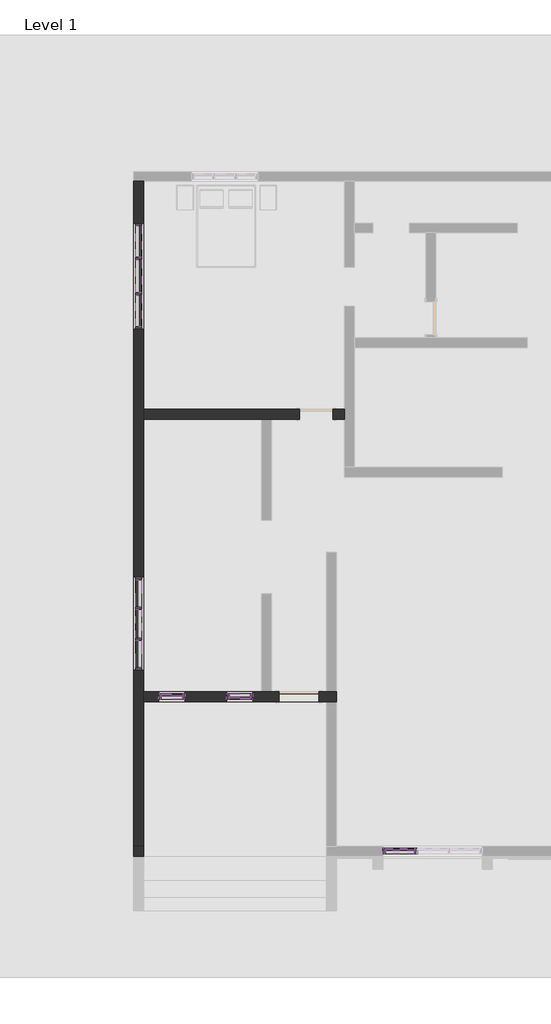
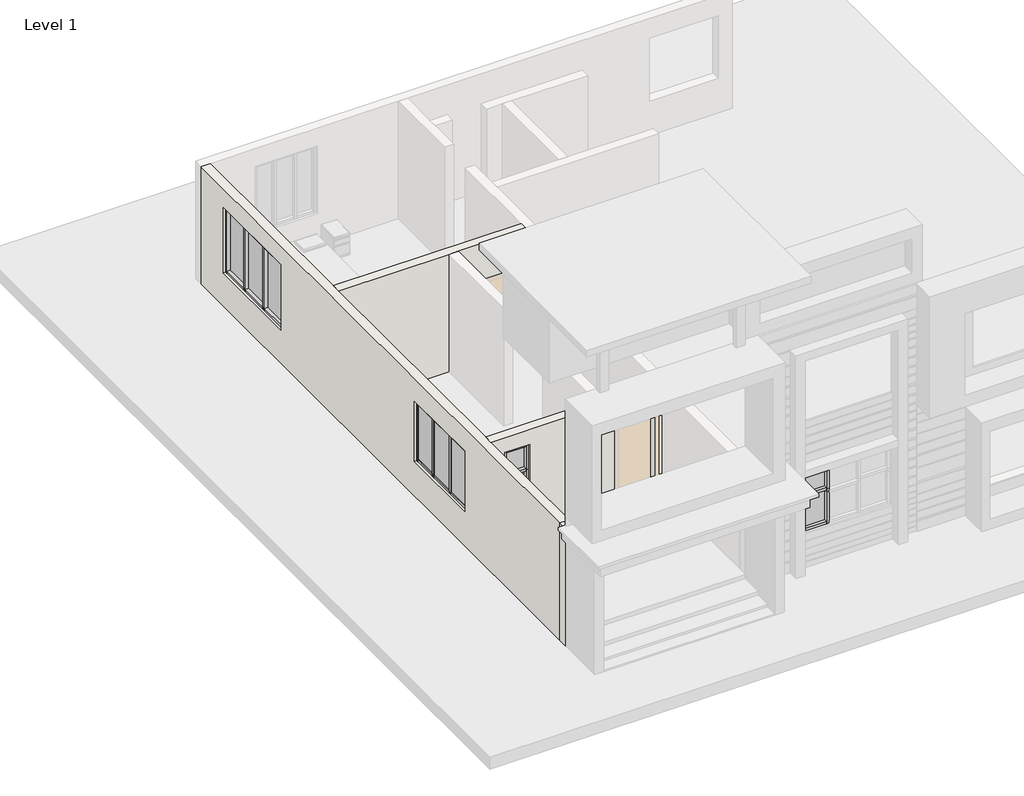
# One storey, part 1 of 3: 49 members, 14 plates, 4 walls.
"""IFC4 building model written with IfcOpenShell, lengths in millimetres."""

from ifc_helpers import new_model, si_unit, origin, origin_with_axes, place, context, project, spatial, polyline, outline, extrude, faceted_brep, transform, mapped, element, save
from components import member_9d02be77, member_7007ad49, member_4a676c08, member_d25e63f8, member_22561c7a, member_3f0e0172, member_607f7529, member_5215b92c, member_00d00b53, member_eb7364f1, member_5ab2641c, member_2ee2964b, member_c33c434a, member_3d7cb871, member_24f36acb, member_a6ee1c2c, member_c4c38143, member_86d06fe4, member_323df77c, member_e6bcc2de, system_panel_glazed_30ed1ba4, system_panel_glazed_23add07f, system_panel_glazed_742ba722, system_panel_glazed_f4631ac9, system_panel_glazed_21711ca4, system_panel_glazed_687c427d, system_panel_glazed_19f1df67, system_panel_glazed_625789f6, system_panel_glazed_f3433a31, system_panel_glazed_9cf13bc3

model = new_model("IFC4")

# Units and contexts
model_context = context("Model", 3, world=origin())
ifc_project = project(units=[si_unit("LENGTHUNIT", "METRE", prefix="MILLI")], contexts=[model_context])

# Site, building, storey
site = spatial("IfcSite", under=ifc_project)
building = spatial("IfcBuilding", under=site)
storey = spatial("IfcBuildingStorey", under=building, Name="Level 1", Elevation=0.0)

# Members
placement = place(None, origin())
member_shape = member_9d02be77(model_context)
element("IfcMember", 1, ObjectType="Rectangular Mullion : 2.5\" x 5\" rectangular", at=placement, inside=storey, context=model_context, shape_type="MappedRepresentation", body=[
    mapped(member_shape, transform((-18686.1761094, -1937.896149, 2567.6785541), x_axis=(0.0, 0.0, 1.0), y_axis=(-1.0, 0.0, 0.0), z_axis=(0.0, -1.0, 0.0))),
])
member_2_shape = member_7007ad49(model_context)
element("IfcMember", 2, ObjectType="Rectangular Mullion : 2.5\" x 5\" rectangular", at=placement, inside=storey, context=model_context, shape_type="MappedRepresentation", body=[
    mapped(member_2_shape, transform((-18686.1761094, -1125.096149, 2567.6785541), x_axis=(0.0, 0.0, 1.0), y_axis=(-1.0, 0.0, 0.0), z_axis=(0.0, -1.0, 0.0))),
])
element("IfcMember", 3, ObjectType="Rectangular Mullion : 2.5\" x 5\" rectangular", at=placement, inside=storey, context=model_context, shape_type="MappedRepresentation", body=[
    mapped(member_2_shape, transform((-18686.1761094, -2718.946149, 2567.6785541), x_axis=(0.0, 0.0, 1.0), y_axis=(-1.0, 0.0, 0.0), z_axis=(0.0, -1.0, 0.0))),
])
member_3_shape = member_4a676c08(model_context)
element("IfcMember", 4, ObjectType="Rectangular Mullion : 2.5\" x 5\" rectangular", at=placement, inside=storey, context=model_context, shape_type="MappedRepresentation", body=[
    mapped(member_3_shape, transform((-18686.1761094, -1969.646149, 870.2260305), x_axis=(0.0, -1.0, 0.0), y_axis=(-1.0, 0.0, 0.0), z_axis=(0.0, 0.0, -1.0))),
])
element("IfcMember", 5, ObjectType="Rectangular Mullion : 2.5\" x 5\" rectangular", at=placement, inside=storey, context=model_context, shape_type="MappedRepresentation", body=[
    mapped(member_3_shape, transform((-18686.1761094, -1156.846149, 870.2260305), x_axis=(0.0, -1.0, 0.0), y_axis=(-1.0, 0.0, 0.0), z_axis=(0.0, 0.0, -1.0))),
])
element("IfcMember", 6, ObjectType="Rectangular Mullion : 2.5\" x 5\" rectangular", at=placement, inside=storey, context=model_context, shape_type="MappedRepresentation", body=[
    mapped(member_2_shape, transform((-18686.1761094, -2001.396149, 870.2260305), x_axis=(0.0, 0.0, -1.0), y_axis=(-1.0, 0.0, 0.0), z_axis=(0.0, 1.0, 0.0))),
])
element("IfcMember", 7, ObjectType="Rectangular Mullion : 2.5\" x 5\" rectangular", at=placement, inside=storey, context=model_context, shape_type="MappedRepresentation", body=[
    mapped(member_2_shape, transform((-18686.1761094, -407.546149, 870.2260305), x_axis=(0.0, 0.0, -1.0), y_axis=(-1.0, 0.0, 0.0), z_axis=(0.0, 1.0, 0.0))),
])
element("IfcMember", 8, ObjectType="Rectangular Mullion : 2.5\" x 5\" rectangular", at=placement, inside=storey, context=model_context, shape_type="MappedRepresentation", body=[
    mapped(member_shape, transform((-18686.1761094, -1188.596149, 870.2260305), x_axis=(0.0, 0.0, -1.0), y_axis=(-1.0, 0.0, 0.0), z_axis=(0.0, 1.0, 0.0))),
])
member_4_shape = member_d25e63f8(model_context)
element("IfcMember", 9, ObjectType="Rectangular Mullion : 2.5\" x 5\" rectangular", at=placement, inside=storey, context=model_context, shape_type="MappedRepresentation", body=[
    mapped(member_4_shape, transform((-18686.1761094, -2782.446149, 870.2260305), x_axis=(0.0, -1.0, 0.0), y_axis=(-1.0, 0.0, 0.0), z_axis=(0.0, 0.0, -1.0))),
])
element("IfcMember", 10, ObjectType="Rectangular Mullion : 2.5\" x 5\" rectangular", at=placement, inside=storey, context=model_context, shape_type="MappedRepresentation", body=[
    mapped(member_4_shape, transform((-18686.1761094, -344.046149, 2567.6785541), x_axis=(0.0, 1.0, 0.0), y_axis=(-1.0, 0.0, 0.0), z_axis=(0.0, 0.0, 1.0))),
])
member_5_shape = member_22561c7a(model_context)
element("IfcMember", 11, ObjectType="Rectangular Mullion : 2.5\" x 5\" rectangular", at=placement, inside=storey, context=model_context, shape_type="MappedRepresentation", body=[
    mapped(member_5_shape, transform((-18686.1761094, -10592.946149, 2458.72085), x_axis=(0.0, -1.0, 0.0), y_axis=(1.0, 0.0, 0.0), z_axis=(0.0, 0.0, 1.0))),
])
member_6_shape = member_3f0e0172(model_context)
element("IfcMember", 12, ObjectType="Rectangular Mullion : 2.5\" x 5\" rectangular", at=placement, inside=storey, context=model_context, shape_type="MappedRepresentation", body=[
    mapped(member_6_shape, transform((-18686.1761094, -9913.496149, 2458.72085), x_axis=(0.0, 0.0, 1.0), y_axis=(1.0, 0.0, 0.0), z_axis=(0.0, 1.0, 0.0))),
])
element("IfcMember", 13, ObjectType="Rectangular Mullion : 2.5\" x 5\" rectangular", at=placement, inside=storey, context=model_context, shape_type="MappedRepresentation", body=[
    mapped(member_6_shape, transform((-18686.1761094, -8522.846149, 2458.72085), x_axis=(0.0, 0.0, 1.0), y_axis=(1.0, 0.0, 0.0), z_axis=(0.0, 1.0, 0.0))),
])
element("IfcMember", 14, ObjectType="Rectangular Mullion : 2.5\" x 5\" rectangular", at=placement, inside=storey, context=model_context, shape_type="MappedRepresentation", body=[
    mapped(member_6_shape, transform((-18686.1761094, -9138.796149, 901.2674751), x_axis=(0.0, 0.0, -1.0), y_axis=(1.0, 0.0, 0.0), z_axis=(0.0, -1.0, 0.0))),
])
element("IfcMember", 15, ObjectType="Rectangular Mullion : 2.5\" x 5\" rectangular", at=placement, inside=storey, context=model_context, shape_type="MappedRepresentation", body=[
    mapped(member_6_shape, transform((-18686.1761094, -10529.446149, 901.2674751), x_axis=(0.0, 0.0, -1.0), y_axis=(1.0, 0.0, 0.0), z_axis=(0.0, -1.0, 0.0))),
])
member_7_shape = member_607f7529(model_context)
element("IfcMember", 16, ObjectType="Rectangular Mullion : 2.5\" x 5\" rectangular", at=placement, inside=storey, context=model_context, shape_type="MappedRepresentation", body=[
    mapped(member_7_shape, transform((-18686.1761094, -9881.746149, 901.2674751), x_axis=(0.0, 1.0, 0.0), y_axis=(1.0, 0.0, 0.0), z_axis=(0.0, 0.0, -1.0))),
])
element("IfcMember", 17, ObjectType="Rectangular Mullion : 2.5\" x 5\" rectangular", at=placement, inside=storey, context=model_context, shape_type="MappedRepresentation", body=[
    mapped(member_7_shape, transform((-18686.1761094, -9170.546149, 901.2674751), x_axis=(0.0, 1.0, 0.0), y_axis=(1.0, 0.0, 0.0), z_axis=(0.0, 0.0, -1.0))),
])
member_8_shape = member_5215b92c(model_context)
element("IfcMember", 18, ObjectType="Rectangular Mullion : 2.5\" x 5\" rectangular", at=placement, inside=storey, context=model_context, shape_type="MappedRepresentation", body=[
    mapped(member_8_shape, transform((-18686.1761094, -9202.296149, 2458.72085), x_axis=(0.0, 0.0, 1.0), y_axis=(1.0, 0.0, 0.0), z_axis=(0.0, 1.0, 0.0))),
])
element("IfcMember", 19, ObjectType="Rectangular Mullion : 2.5\" x 5\" rectangular", at=placement, inside=storey, context=model_context, shape_type="MappedRepresentation", body=[
    mapped(member_8_shape, transform((-18686.1761094, -9849.996149, 901.2674751), x_axis=(0.0, 0.0, -1.0), y_axis=(1.0, 0.0, 0.0), z_axis=(0.0, -1.0, 0.0))),
])
element("IfcMember", 20, ObjectType="Rectangular Mullion : 2.5\" x 5\" rectangular", at=placement, inside=storey, context=model_context, shape_type="MappedRepresentation", body=[
    mapped(member_5_shape, transform((-18686.1761094, -8459.346149, 901.2674751), x_axis=(0.0, 1.0, 0.0), y_axis=(1.0, 0.0, 0.0), z_axis=(0.0, 0.0, -1.0))),
])
member_9_shape = member_00d00b53(model_context)
element("IfcMember", 21, ObjectType="Rectangular Mullion : 2.5\" x 5\" rectangular", at=placement, inside=storey, context=model_context, shape_type="MappedRepresentation", body=[
    mapped(member_9_shape, transform((-12323.9127168, -14745.846149, 1704.2081862), x_axis=(1.0, 0.0, 0.0), y_axis=(0.0, -1.0, 0.0), z_axis=(0.0, 0.0, -1.0))),
])
member_10_shape = member_eb7364f1(model_context)
element("IfcMember", 22, ObjectType="Rectangular Mullion : 2.5\" x 5\" rectangular", at=placement, inside=storey, context=model_context, shape_type="MappedRepresentation", body=[
    mapped(member_10_shape, transform((-12323.9127168, -14745.846149, 1780.4081862), x_axis=(1.0, 0.0, 0.0), y_axis=(0.0, -1.0, 0.0), z_axis=(0.0, 0.0, -1.0))),
])
member_11_shape = member_5ab2641c(model_context)
element("IfcMember", 23, ObjectType="Rectangular Mullion : 2.5\" x 5\" rectangular", at=placement, inside=storey, context=model_context, shape_type="MappedRepresentation", body=[
    mapped(member_11_shape, transform((-12323.9127168, -14745.846149, 871.6720769), x_axis=(1.0, 0.0, 0.0), y_axis=(0.0, -1.0, 0.0), z_axis=(0.0, 0.0, -1.0))),
])
member_12_shape = member_2ee2964b(model_context)
element("IfcMember", 24, ObjectType="Rectangular Mullion : 2.5\" x 5\" rectangular", at=placement, inside=storey, context=model_context, shape_type="MappedRepresentation", body=[
    mapped(member_12_shape, transform((-12355.6627168, -14745.846149, 1780.4081862), x_axis=(0.0, 0.0, 1.0), y_axis=(0.0, -1.0, 0.0), z_axis=(1.0, 0.0, 0.0))),
])
member_13_shape = member_c33c434a(model_context)
element("IfcMember", 25, ObjectType="Rectangular Mullion : 2.5\" x 5\" rectangular", at=placement, inside=storey, context=model_context, shape_type="MappedRepresentation", body=[
    mapped(member_13_shape, transform((-12355.6627168, -14745.846149, 2536.7442955), x_axis=(0.0, 0.0, 1.0), y_axis=(0.0, -1.0, 0.0), z_axis=(1.0, 0.0, 0.0))),
])
element("IfcMember", 26, ObjectType="Rectangular Mullion : 2.5\" x 5\" rectangular", at=placement, inside=storey, context=model_context, shape_type="MappedRepresentation", body=[
    mapped(member_13_shape, transform((-13022.4127168, -14745.846149, 871.6720769), x_axis=(0.0, 0.0, -1.0), y_axis=(0.0, -1.0, 0.0), z_axis=(-1.0, 0.0, 0.0))),
])
member_14_shape = member_3d7cb871(model_context)
element("IfcMember", 27, ObjectType="Rectangular Mullion : 2.5\" x 5\" rectangular", at=placement, inside=storey, context=model_context, shape_type="MappedRepresentation", body=[
    mapped(member_14_shape, transform((-13085.9127168, -14745.846149, 1780.4081862), x_axis=(-1.0, 0.0, 0.0), y_axis=(0.0, -1.0, 0.0), z_axis=(0.0, 0.0, 1.0))),
])
member_15_shape = member_24f36acb(model_context)
element("IfcMember", 28, ObjectType="Rectangular Mullion : 2.5\" x 5\" rectangular", at=placement, inside=storey, context=model_context, shape_type="MappedRepresentation", body=[
    mapped(member_15_shape, transform((-13085.9127168, -14745.846149, 1704.2081862), x_axis=(-1.0, 0.0, 0.0), y_axis=(0.0, -1.0, 0.0), z_axis=(0.0, 0.0, 1.0))),
])
member_16_shape = member_a6ee1c2c(model_context)
element("IfcMember", 29, ObjectType="Rectangular Mullion : 2.5\" x 5\" rectangular", at=placement, inside=storey, context=model_context, shape_type="MappedRepresentation", body=[
    mapped(member_16_shape, transform((-13085.9127168, -14745.846149, 2536.7442955), x_axis=(-1.0, 0.0, 0.0), y_axis=(0.0, -1.0, 0.0), z_axis=(0.0, 0.0, 1.0))),
])
member_17_shape = member_c4c38143(model_context)
element("IfcMember", 30, ObjectType="Rectangular Mullion : 2.5\" x 5\" rectangular", at=placement, inside=storey, context=model_context, shape_type="MappedRepresentation", body=[
    mapped(member_17_shape, transform((-16057.2761094, -11202.546149, 2600.4840587), x_axis=(1.0, 0.0, 0.0), y_axis=(0.0, 1.0, 0.0), z_axis=(0.0, 0.0, 1.0))),
])
member_18_shape = member_86d06fe4(model_context)
element("IfcMember", 31, ObjectType="Rectangular Mullion : 2.5\" x 5\" rectangular", at=placement, inside=storey, context=model_context, shape_type="MappedRepresentation", body=[
    mapped(member_18_shape, transform((-16603.3761094, -11202.546149, 2600.4840587), x_axis=(0.0, 0.0, 1.0), y_axis=(0.0, 1.0, 0.0), z_axis=(-1.0, 0.0, 0.0))),
])
element("IfcMember", 32, ObjectType="Rectangular Mullion : 2.5\" x 5\" rectangular", at=placement, inside=storey, context=model_context, shape_type="MappedRepresentation", body=[
    mapped(member_18_shape, transform((-17682.8761094, -11202.546149, 2660.8518788), x_axis=(0.0, 0.0, 1.0), y_axis=(0.0, -1.0, 0.0), z_axis=(1.0, 0.0, 0.0))),
])
member_19_shape = member_323df77c(model_context)
element("IfcMember", 33, ObjectType="Rectangular Mullion : 2.5\" x 5\" rectangular", at=placement, inside=storey, context=model_context, shape_type="MappedRepresentation", body=[
    mapped(member_19_shape, transform((-16603.3761094, -11202.546149, 1942.3889092), x_axis=(0.0, 0.0, 1.0), y_axis=(0.0, 1.0, 0.0), z_axis=(-1.0, 0.0, 0.0))),
])
element("IfcMember", 34, ObjectType="Rectangular Mullion : 2.5\" x 5\" rectangular", at=placement, inside=storey, context=model_context, shape_type="MappedRepresentation", body=[
    mapped(member_19_shape, transform((-16603.3761094, -11202.546149, 1284.2937596), x_axis=(0.0, 0.0, 1.0), y_axis=(0.0, 1.0, 0.0), z_axis=(-1.0, 0.0, 0.0))),
])
element("IfcMember", 35, ObjectType="Rectangular Mullion : 2.5\" x 5\" rectangular", at=placement, inside=storey, context=model_context, shape_type="MappedRepresentation", body=[
    mapped(member_19_shape, transform((-17682.8761094, -11202.546149, 1995.3876199), x_axis=(0.0, 0.0, 1.0), y_axis=(0.0, -1.0, 0.0), z_axis=(1.0, 0.0, 0.0))),
])
element("IfcMember", 36, ObjectType="Rectangular Mullion : 2.5\" x 5\" rectangular", at=placement, inside=storey, context=model_context, shape_type="MappedRepresentation", body=[
    mapped(member_19_shape, transform((-17682.8761094, -11202.546149, 1329.923361), x_axis=(0.0, 0.0, 1.0), y_axis=(0.0, -1.0, 0.0), z_axis=(1.0, 0.0, 0.0))),
])
element("IfcMember", 37, ObjectType="Rectangular Mullion : 2.5\" x 5\" rectangular", at=placement, inside=storey, context=model_context, shape_type="MappedRepresentation", body=[
    mapped(member_17_shape, transform((-16666.8761094, -11202.546149, 1942.3889092), x_axis=(-1.0, 0.0, 0.0), y_axis=(0.0, 1.0, 0.0), z_axis=(0.0, 0.0, -1.0))),
])
element("IfcMember", 38, ObjectType="Rectangular Mullion : 2.5\" x 5\" rectangular", at=placement, inside=storey, context=model_context, shape_type="MappedRepresentation", body=[
    mapped(member_17_shape, transform((-16057.2761094, -11202.546149, 1942.3889092), x_axis=(1.0, 0.0, 0.0), y_axis=(0.0, 1.0, 0.0), z_axis=(0.0, 0.0, 1.0))),
])
element("IfcMember", 39, ObjectType="Rectangular Mullion : 2.5\" x 5\" rectangular", at=placement, inside=storey, context=model_context, shape_type="MappedRepresentation", body=[
    mapped(member_17_shape, transform((-16666.8761094, -11202.546149, 1284.2937596), x_axis=(-1.0, 0.0, 0.0), y_axis=(0.0, 1.0, 0.0), z_axis=(0.0, 0.0, -1.0))),
])
element("IfcMember", 40, ObjectType="Rectangular Mullion : 2.5\" x 5\" rectangular", at=placement, inside=storey, context=model_context, shape_type="MappedRepresentation", body=[
    mapped(member_18_shape, transform((-16120.7761094, -11202.546149, 626.1986101), x_axis=(0.0, 0.0, -1.0), y_axis=(0.0, 1.0, 0.0), z_axis=(1.0, 0.0, 0.0))),
])
element("IfcMember", 41, ObjectType="Rectangular Mullion : 2.5\" x 5\" rectangular", at=placement, inside=storey, context=model_context, shape_type="MappedRepresentation", body=[
    mapped(member_18_shape, transform((-18165.4761094, -11202.546149, 664.4591022), x_axis=(0.0, 0.0, -1.0), y_axis=(0.0, -1.0, 0.0), z_axis=(-1.0, 0.0, 0.0))),
])
element("IfcMember", 42, ObjectType="Rectangular Mullion : 2.5\" x 5\" rectangular", at=placement, inside=storey, context=model_context, shape_type="MappedRepresentation", body=[
    mapped(member_17_shape, transform((-16057.2761094, -11202.546149, 1284.2937596), x_axis=(1.0, 0.0, 0.0), y_axis=(0.0, 1.0, 0.0), z_axis=(0.0, 0.0, 1.0))),
])
element("IfcMember", 43, ObjectType="Rectangular Mullion : 2.5\" x 5\" rectangular", at=placement, inside=storey, context=model_context, shape_type="MappedRepresentation", body=[
    mapped(member_17_shape, transform((-16666.8761094, -11202.546149, 626.1986101), x_axis=(-1.0, 0.0, 0.0), y_axis=(0.0, 1.0, 0.0), z_axis=(0.0, 0.0, -1.0))),
])
member_20_shape = member_e6bcc2de(model_context)
element("IfcMember", 44, ObjectType="Rectangular Mullion : 2.5\" x 5\" rectangular", at=placement, inside=storey, context=model_context, shape_type="MappedRepresentation", body=[
    mapped(member_20_shape, transform((-17619.3761094, -11202.546149, 1995.3876199), x_axis=(1.0, 0.0, 0.0), y_axis=(0.0, -1.0, 0.0), z_axis=(0.0, 0.0, -1.0))),
])
element("IfcMember", 45, ObjectType="Rectangular Mullion : 2.5\" x 5\" rectangular", at=placement, inside=storey, context=model_context, shape_type="MappedRepresentation", body=[
    mapped(member_20_shape, transform((-17619.3761094, -11202.546149, 1329.923361), x_axis=(1.0, 0.0, 0.0), y_axis=(0.0, -1.0, 0.0), z_axis=(0.0, 0.0, -1.0))),
])
element("IfcMember", 46, ObjectType="Rectangular Mullion : 2.5\" x 5\" rectangular", at=placement, inside=storey, context=model_context, shape_type="MappedRepresentation", body=[
    mapped(member_20_shape, transform((-18228.9761094, -11202.546149, 1995.3876199), x_axis=(-1.0, 0.0, 0.0), y_axis=(0.0, -1.0, 0.0), z_axis=(0.0, 0.0, 1.0))),
])
element("IfcMember", 47, ObjectType="Rectangular Mullion : 2.5\" x 5\" rectangular", at=placement, inside=storey, context=model_context, shape_type="MappedRepresentation", body=[
    mapped(member_20_shape, transform((-18228.9761094, -11202.546149, 2660.8518788), x_axis=(-1.0, 0.0, 0.0), y_axis=(0.0, -1.0, 0.0), z_axis=(0.0, 0.0, 1.0))),
])
element("IfcMember", 48, ObjectType="Rectangular Mullion : 2.5\" x 5\" rectangular", at=placement, inside=storey, context=model_context, shape_type="MappedRepresentation", body=[
    mapped(member_20_shape, transform((-17619.3761094, -11202.546149, 664.4591022), x_axis=(1.0, 0.0, 0.0), y_axis=(0.0, -1.0, 0.0), z_axis=(0.0, 0.0, -1.0))),
])
element("IfcMember", 49, ObjectType="Rectangular Mullion : 2.5\" x 5\" rectangular", at=placement, inside=storey, context=model_context, shape_type="MappedRepresentation", body=[
    mapped(member_20_shape, transform((-18228.9761094, -11202.546149, 1329.923361), x_axis=(-1.0, 0.0, 0.0), y_axis=(0.0, -1.0, 0.0), z_axis=(0.0, 0.0, 1.0))),
])

# Plates
system_panel_glazed_shape = system_panel_glazed_30ed1ba4(model_context)
element("IfcPlate", 50, ObjectType="System Panel : Glazed", at=placement, inside=storey, context=model_context, shape_type="MappedRepresentation", body=[
    mapped(system_panel_glazed_shape, transform((-18686.1761094, -766.321149, 933.7260305), x_axis=(0.0, -1.0, 0.0), y_axis=(1.0, 0.0, 0.0), z_axis=(0.0, 0.0, 1.0))),
])
element("IfcPlate", 51, ObjectType="System Panel : Glazed", at=placement, inside=storey, context=model_context, shape_type="MappedRepresentation", body=[
    mapped(system_panel_glazed_shape, transform((-18686.1761094, -2360.171149, 933.7260305), x_axis=(0.0, -1.0, 0.0), y_axis=(1.0, 0.0, 0.0), z_axis=(0.0, 0.0, 1.0))),
])
system_panel_glazed_2_shape = system_panel_glazed_23add07f(model_context)
element("IfcPlate", 52, ObjectType="System Panel : Glazed", at=placement, inside=storey, context=model_context, shape_type="MappedRepresentation", body=[
    mapped(system_panel_glazed_2_shape, transform((-18686.1761094, -1563.246149, 933.7260305), x_axis=(0.0, -1.0, 0.0), y_axis=(1.0, 0.0, 0.0), z_axis=(0.0, 0.0, 1.0))),
])
system_panel_glazed_3_shape = system_panel_glazed_742ba722(model_context)
element("IfcPlate", 53, ObjectType="System Panel : Glazed", at=placement, inside=storey, context=model_context, shape_type="MappedRepresentation", body=[
    mapped(system_panel_glazed_3_shape, transform((-18686.1761094, -10221.471149, 964.7674751), x_axis=(0.0, 1.0, 0.0), y_axis=(-1.0, 0.0, 0.0), z_axis=(0.0, 0.0, 1.0))),
])
element("IfcPlate", 54, ObjectType="System Panel : Glazed", at=placement, inside=storey, context=model_context, shape_type="MappedRepresentation", body=[
    mapped(system_panel_glazed_3_shape, transform((-18686.1761094, -8830.821149, 964.7674751), x_axis=(0.0, 1.0, 0.0), y_axis=(-1.0, 0.0, 0.0), z_axis=(0.0, 0.0, 1.0))),
])
system_panel_glazed_4_shape = system_panel_glazed_f4631ac9(model_context)
element("IfcPlate", 55, ObjectType="System Panel : Glazed", at=placement, inside=storey, context=model_context, shape_type="MappedRepresentation", body=[
    mapped(system_panel_glazed_4_shape, transform((-18686.1761094, -9526.146149, 964.7674751), x_axis=(0.0, 1.0, 0.0), y_axis=(-1.0, 0.0, 0.0), z_axis=(0.0, 0.0, 1.0))),
])
system_panel_glazed_5_shape = system_panel_glazed_21711ca4(model_context)
element("IfcPlate", 56, ObjectType="System Panel : Glazed", at=placement, inside=storey, context=model_context, shape_type="MappedRepresentation", body=[
    mapped(system_panel_glazed_5_shape, transform((-12689.0377168, -14745.846149, 935.1720769), x_axis=(1.0, 0.0, 0.0), y_axis=(0.0, 1.0, 0.0), z_axis=(0.0, 0.0, 1.0))),
])
system_panel_glazed_6_shape = system_panel_glazed_687c427d(model_context)
element("IfcPlate", 57, ObjectType="System Panel : Glazed", at=placement, inside=storey, context=model_context, shape_type="MappedRepresentation", body=[
    mapped(system_panel_glazed_6_shape, transform((-12689.0377168, -14745.846149, 1812.1581862), x_axis=(1.0, 0.0, 0.0), y_axis=(0.0, 1.0, 0.0), z_axis=(0.0, 0.0, 1.0))),
])
system_panel_glazed_7_shape = system_panel_glazed_19f1df67(model_context)
element("IfcPlate", 58, ObjectType="System Panel : Glazed", at=placement, inside=storey, context=model_context, shape_type="MappedRepresentation", body=[
    mapped(system_panel_glazed_7_shape, transform((-16362.0761094, -11202.546149, 689.6986101), x_axis=(-1.0, 0.0, 0.0), y_axis=(0.0, -1.0, 0.0), z_axis=(0.0, 0.0, 1.0))),
])
element("IfcPlate", 59, ObjectType="System Panel : Glazed", at=placement, inside=storey, context=model_context, shape_type="MappedRepresentation", body=[
    mapped(system_panel_glazed_7_shape, transform((-16362.0761094, -11202.546149, 1974.1389092), x_axis=(-1.0, 0.0, 0.0), y_axis=(0.0, -1.0, 0.0), z_axis=(0.0, 0.0, 1.0))),
])
system_panel_glazed_8_shape = system_panel_glazed_625789f6(model_context)
element("IfcPlate", 60, ObjectType="System Panel : Glazed", at=placement, inside=storey, context=model_context, shape_type="MappedRepresentation", body=[
    mapped(system_panel_glazed_8_shape, transform((-16362.0761094, -11202.546149, 1316.0437596), x_axis=(-1.0, 0.0, 0.0), y_axis=(0.0, -1.0, 0.0), z_axis=(0.0, 0.0, 1.0))),
])
system_panel_glazed_9_shape = system_panel_glazed_f3433a31(model_context)
element("IfcPlate", 61, ObjectType="System Panel : Glazed", at=placement, inside=storey, context=model_context, shape_type="MappedRepresentation", body=[
    mapped(system_panel_glazed_9_shape, transform((-17924.1761094, -11202.546149, 727.9591022), x_axis=(1.0, 0.0, 0.0), y_axis=(0.0, 1.0, 0.0), z_axis=(0.0, 0.0, 1.0))),
])
element("IfcPlate", 62, ObjectType="System Panel : Glazed", at=placement, inside=storey, context=model_context, shape_type="MappedRepresentation", body=[
    mapped(system_panel_glazed_9_shape, transform((-17924.1761094, -11202.546149, 2027.1376199), x_axis=(1.0, 0.0, 0.0), y_axis=(0.0, 1.0, 0.0), z_axis=(0.0, 0.0, 1.0))),
])
system_panel_glazed_10_shape = system_panel_glazed_9cf13bc3(model_context)
element("IfcPlate", 63, ObjectType="System Panel : Glazed", at=placement, inside=storey, context=model_context, shape_type="MappedRepresentation", body=[
    mapped(system_panel_glazed_10_shape, transform((-17924.1761094, -11202.546149, 1361.673361), x_axis=(1.0, 0.0, 0.0), y_axis=(0.0, 1.0, 0.0), z_axis=(0.0, 0.0, 1.0))),
])

# Walls
element("IfcWall", 64, ObjectType="9\"", at=placement, inside=storey, context=model_context, shape_type="SweptSolid", body=[
    extrude(outline(polyline([(-18571.8761094, -14860.146149), (-18800.4761094, -14860.146149), (-18800.4761094, -14631.546149), (-18571.8761094, -14631.546149), (-18571.8761094, -14860.146149)])), origin_with_axes(), (0.0, 0.0, 1.0), 3048.0),
])
element("IfcWall", 65, ObjectType="9\"", at=placement, inside=storey, context=model_context, shape_type="Brep", body=[
    faceted_brep([(-18800.4761094, 608.453851, 0.0), (-18800.4761094, -14631.546149, 0.0), (-18800.4761094, -14631.546149, 3048.0), (-18800.4761094, 608.453851, 3048.0), (-18800.4761094, -344.046149, 870.2260305), (-18800.4761094, -344.046149, 2567.6785541), (-18800.4761094, -2782.446149, 2567.6785541), (-18800.4761094, -2782.446149, 870.2260305), (-18800.4761094, -10592.946149, 2458.72085), (-18800.4761094, -10592.946149, 901.2674751), (-18800.4761094, -8459.346149, 901.2674751), (-18800.4761094, -8459.346149, 2458.72085), (-18571.8761094, -14631.546149, 0.0), (-18571.8761094, -11316.846149, 0.0), (-18571.8761094, -11088.246149, 0.0), (-18571.8761094, -4839.846149, 0.0), (-18571.8761094, -4611.246149, 0.0), (-18571.8761094, 608.453851, 0.0), (-18571.8761094, 608.453851, 3048.0), (-18571.8761094, -4611.246149, 3048.0), (-18571.8761094, -4839.846149, 3048.0), (-18571.8761094, -11088.246149, 3048.0), (-18571.8761094, -11316.846149, 3048.0), (-18571.8761094, -14631.546149, 3048.0), (-18571.8761094, -344.046149, 2567.6785541), (-18571.8761094, -344.046149, 870.2260305), (-18571.8761094, -2782.446149, 870.2260305), (-18571.8761094, -2782.446149, 2567.6785541), (-18571.8761094, -10592.946149, 901.2674751), (-18571.8761094, -10592.946149, 2458.72085), (-18571.8761094, -8459.346149, 2458.72085), (-18571.8761094, -8459.346149, 901.2674751)], [[[0, 1, 2, 3], [4, 5, 6, 7], [8, 9, 10, 11]], [[12, 13, 14, 15, 16, 17, 18, 19, 20, 21, 22, 23], [24, 25, 26, 27], [28, 29, 30, 31]], [[1, 0, 17, 16, 15, 14, 13, 12]], [[3, 2, 23, 22, 21, 20, 19, 18]], [[0, 3, 18, 17]], [[2, 1, 12, 23]], [[24, 5, 4, 25]], [[5, 24, 27, 6]], [[6, 27, 26, 7]], [[25, 4, 7, 26]], [[28, 9, 8, 29]], [[29, 8, 11, 30]], [[30, 11, 10, 31]], [[9, 28, 31, 10]]]),
])
element("IfcWall", 66, ObjectType="9\"", at=placement, inside=storey, context=model_context, shape_type="Brep", body=[
    faceted_brep([(-18571.8761094, -11316.846149, 0.0), (-14380.8761094, -11316.846149, 0.0), (-14152.2761094, -11316.846149, 0.0), (-14152.2761094, -11316.846149, 3048.0), (-14380.8761094, -11316.846149, 3048.0), (-18571.8761094, -11316.846149, 3048.0), (-14552.3261094, -11316.846149, 355.6), (-15466.7261094, -11316.846149, 355.6), (-15466.7261094, -11316.846149, 2489.2), (-14552.3261094, -11316.846149, 2489.2), (-16057.2761094, -11316.846149, 2600.4840587), (-16057.2761094, -11316.846149, 626.1986101), (-16666.8761094, -11316.846149, 626.1986101), (-16666.8761094, -11316.846149, 2600.4840587), (-18228.9761094, -11316.846149, 664.4591022), (-18228.9761094, -11316.846149, 2660.8518788), (-17619.3761094, -11316.846149, 2660.8518788), (-17619.3761094, -11316.846149, 664.4591022), (-14152.2761094, -11088.246149, 0.0), (-14380.8761094, -11088.246149, 0.0), (-15638.1761094, -11088.246149, 0.0), (-15866.7761094, -11088.246149, 0.0), (-18571.8761094, -11088.246149, 0.0), (-18571.8761094, -11088.246149, 3048.0), (-15866.7761094, -11088.246149, 3048.0), (-15638.1761094, -11088.246149, 3048.0), (-14380.8761094, -11088.246149, 3048.0), (-14152.2761094, -11088.246149, 3048.0), (-15466.7261094, -11088.246149, 355.6), (-14552.3261094, -11088.246149, 355.6), (-14552.3261094, -11088.246149, 2489.2), (-15466.7261094, -11088.246149, 2489.2), (-16057.2761094, -11088.246149, 626.1986101), (-16057.2761094, -11088.246149, 2600.4840587), (-16666.8761094, -11088.246149, 2600.4840587), (-16666.8761094, -11088.246149, 626.1986101), (-18228.9761094, -11088.246149, 2660.8518788), (-18228.9761094, -11088.246149, 664.4591022), (-17619.3761094, -11088.246149, 664.4591022), (-17619.3761094, -11088.246149, 2660.8518788)], [[[0, 1, 2, 3, 4, 5], [6, 7, 8, 9], [10, 11, 12, 13], [14, 15, 16, 17]], [[18, 19, 20, 21, 22, 23, 24, 25, 26, 27], [28, 29, 30, 31], [32, 33, 34, 35], [36, 37, 38, 39]], [[2, 1, 0, 22, 21, 20, 19, 18]], [[5, 4, 3, 27, 26, 25, 24, 23]], [[0, 5, 23, 22]], [[3, 2, 18, 27]], [[29, 28, 7, 6]], [[30, 29, 6, 9]], [[31, 30, 9, 8]], [[28, 31, 8, 7]], [[32, 11, 10, 33]], [[33, 10, 13, 34]], [[34, 13, 12, 35]], [[11, 32, 35, 12]], [[36, 15, 14, 37]], [[15, 36, 39, 16]], [[16, 39, 38, 17]], [[37, 14, 17, 38]]]),
])
element("IfcWall", 67, ObjectType="9\"", at=placement, inside=storey, context=model_context, shape_type="Brep", body=[
    faceted_brep([(-13962.2127168, -4611.246149, 0.0), (-14228.9127168, -4611.246149, 0.0), (-14228.9127168, -4611.246149, 2032.0), (-14990.9127168, -4611.246149, 2032.0), (-14990.9127168, -4611.246149, 0.0), (-18571.8761094, -4611.246149, 0.0), (-18571.8761094, -4611.246149, 3048.0), (-13962.2127168, -4611.246149, 3048.0), (-14228.9127168, -4839.846149, 2032.0), (-14228.9127168, -4839.846149, 0.0), (-13962.2127168, -4839.846149, 0.0), (-13962.2127168, -4839.846149, 3048.0), (-15638.1761094, -4839.846149, 3048.0), (-15866.7761094, -4839.846149, 3048.0), (-18571.8761094, -4839.846149, 3048.0), (-18571.8761094, -4839.846149, 0.0), (-15866.7761094, -4839.846149, 0.0), (-15638.1761094, -4839.846149, 0.0), (-14990.9127168, -4839.846149, 0.0), (-14990.9127168, -4839.846149, 2032.0)], [[[0, 1, 2, 3, 4, 5, 6, 7]], [[8, 9, 10, 11, 12, 13, 14, 15, 16, 17, 18, 19]], [[10, 9, 1, 0]], [[18, 17, 16, 15, 5, 4]], [[7, 6, 14, 13, 12, 11]], [[6, 5, 15, 14]], [[0, 7, 11, 10]], [[2, 1, 9, 8]], [[3, 2, 8, 19]], [[4, 3, 19, 18]]]),
])

save(model, "model.ifc")

# Revit data of these elements
# Type "Rectangular Mullion : 2.5\" x 5\" rectangular"
#   built-in parameter 1007304 = 0.416667 (stored number, unit not read)
#   built-in parameter 1007301 = 0.104167 (stored number, unit not read)
#   built-in parameter 1007300 = 0.104167 (stored number, unit not read)
# Type "System Panel : Glazed"
#   Construction Type Id = "GSP4R"
#   Analytic Construction = "1/8 in Pilkington single glazing"
#   Visual Light Transmittance = 0.9
#   Solar Heat Gain Coefficient = 0.86
#   Heat Transfer Coefficient (U) = 1.18115 BTU/(h·ft²·°F)
#   Define Thermal Properties by = 1
# Type "9\""
#   Assembly Code = "B2010"
#   Layers, outside or top first: 0' - 9" no material (function 1)
# Elements 1, 2, 3, 4, 5, 6, 7, 8, 9, 10, 11, 12, 13, 14, 15, 16, 17, 18, 19, 20, 21, 22, 23, 24, 25, 26, 27, 28, 29, 30, 31, 32, 33, 34, 35, 36, 37, 38, 39, 40, 41, 42, 43, 44, 45, 46, 47, 48, 49 (IfcMember, "Rectangular Mullion : 2.5\" x 5\" rectangular")
#   Phase Created = New Construction
#   Materials on its faces: "Aluminum"
# Elements 50, 51, 52, 53, 54, 55, 56, 57, 58, 59, 60, 61, 62, 63 (IfcPlate, "System Panel : Glazed")
#   Phase Created = New Construction
#   Materials on its faces: "Glass"
# Elements 64, 65, 66, 67 (IfcWall, "9\"")
#   Top Offset = 0' - 0"
#   Base Offset = 0' - 0"
#   Unconnected Height = 10' - 0"
#   wall height = 10' - 0"
#   Phase Created = New Construction
#   Base Constraint = Level 1
#   Materials on its faces: "Default Wall"
# Materials
#   "Aluminum": class "Metal", colour RGB 247 247 247, transparency 0, Description = "Aluminum 6061", Cost = 0
#   "Glass": class "Glass", colour RGB 0 128 192, transparency 0.75, Description = "Soda Lime Glass", Cost = 0
#   "Default Wall": colour RGB 128 128 128, transparency 0, Cost = 0
